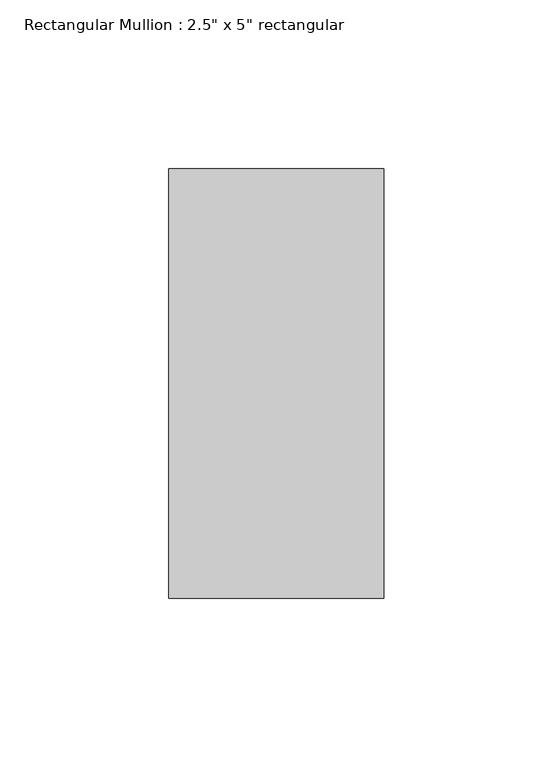
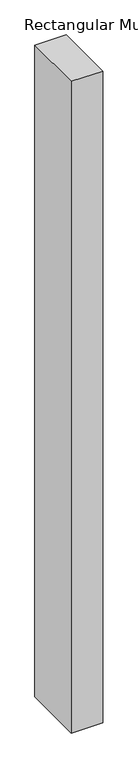
"""IFC4 building model written with IfcOpenShell, lengths in millimetres: member geometry."""

from ifc_helpers import new_model, si_unit, frame, origin, place, context, project, spatial, polyline, outline, extrude, source, transform, mapped, element, save


def member_fcbfb253(model_context):
    return source(origin(), model_context, "Body", "SweptSolid", [
        extrude(outline(polyline([(31.75, 63.5), (31.75, -63.5), (-31.75, -63.5), (-31.75, 63.5), (31.75, 63.5)])), frame((0.0, 0.0, -1388.8321364), z_axis=(0.0, 0.0, 1.0), x_axis=(1.0, 0.0, 0.0)), (0.0, 0.0, 1.0), 1388.8321364),
    ])


if __name__ == "__main__":
    model = new_model("IFC4")
    model_context = context("Model", 3, world=origin())
    ifc_project = project(units=[si_unit("LENGTHUNIT", "METRE", prefix="MILLI")], contexts=[model_context])
    site = spatial("IfcSite", under=ifc_project)
    building = spatial("IfcBuilding", under=site)
    placement = place(None, origin())
    member_shape = member_fcbfb253(model_context)
    element("IfcMember", 1, ObjectType="Rectangular Mullion : 2.5\" x 5\" rectangular", at=placement, inside=building, context=model_context, shape_type="MappedRepresentation", body=[
        mapped(member_shape, transform((0.0, 0.0, 0.0), x_axis=(1.0, 0.0, 0.0), y_axis=(0.0, 1.0, 0.0), z_axis=(0.0, 0.0, 1.0))),
    ])
    save(model, "model.ifc")

# Revit data of these elements
# Type "Rectangular Mullion : 2.5\" x 5\" rectangular"
#   built-in parameter 1007304 = 0.416667 (stored number, unit not read)
#   built-in parameter 1007301 = 0.104167 (stored number, unit not read)
#   built-in parameter 1007300 = 0.104167 (stored number, unit not read)
# Element 1 (IfcMember, "Rectangular Mullion : 2.5\" x 5\" rectangular")
#   Materials on its faces: "Aluminum"
# Materials
#   "Aluminum": class "Metal", colour RGB 247 247 247, transparency 0, Description = "Aluminum 6061", Cost = 0
